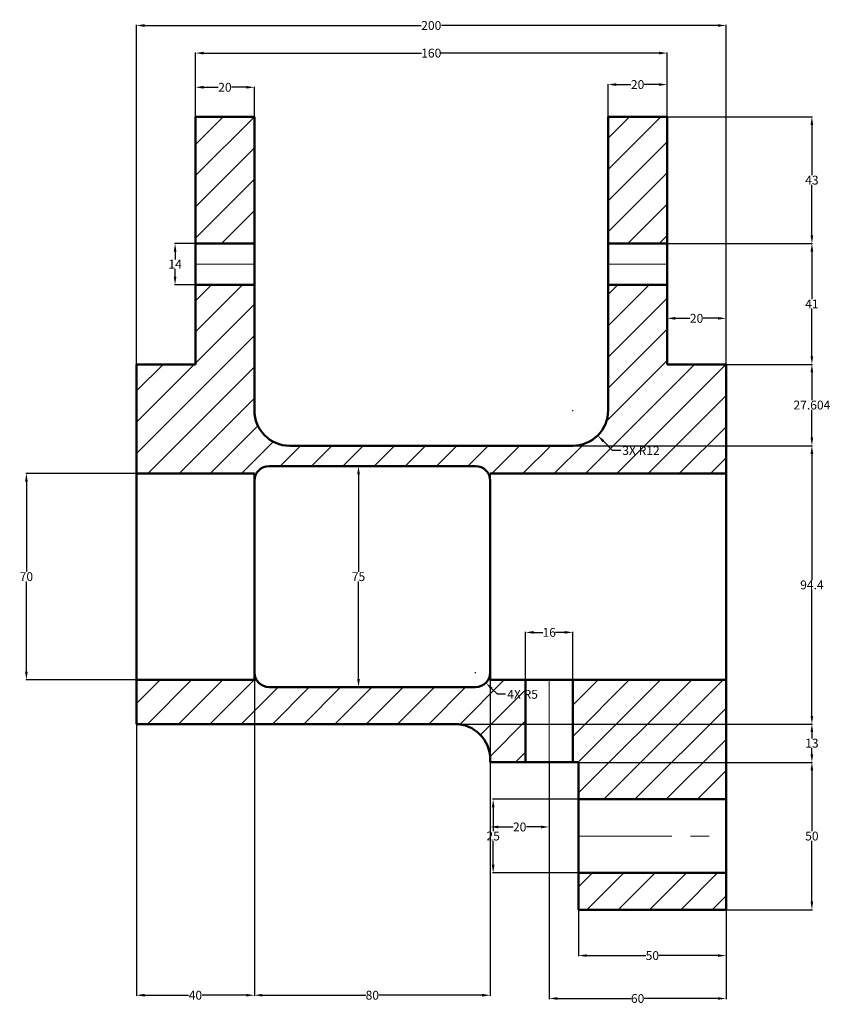
# Model space of a CAD drawing. Units: millimetres. Extents: x 164 to 765, y 152 to 486.
# Tile 2 of 2: x 490 to 765, y 152 to 486. Entities that reach past the tile are written whole.
import ezdxf

# ---------------------------------------------------------------- set-up
doc = ezdxf.new("R2010")
doc.units = ezdxf.units.MM
doc.header["$MEASUREMENT"] = 0
doc.linetypes.add('CENTER', pattern=[50.8, 31.75, -6.35, 6.35, -6.35])
for name, color, linetype, lineweight in [('M-CNTR', 1, 'CENTER', 18), ('M-DIMS', 2, 'Continuous', 25), ('M-HATC', 8, 'Continuous', 18), ('M-OUTL', 7, 'Continuous', 50)]:
    doc.layers.add(name, color=color, linetype=linetype, lineweight=lineweight)
doc.styles.get("Standard").update_dxf_attribs({"font": 'arial.ttf'})
doc.dimstyles.get("Standard").update_dxf_attribs({"dimtxt": 3, "dimasz": 2.75, "dimexe": 0.18, "dimexo": 0.0625, "dimgap": 0.09, "dimtad": 0, "dimtih": 1, "dimtoh": 1, "dimdec": 0, "dimzin": 0, "dimdsep": 46, "dimtxsty": 'Standard', "dimcen": 0.09, "dimadec": 0, "dimazin": 0, "dimtfac": 1, "dimtdec": 0, "dimtofl": 0, "dimtmove": 0, "dimatfit": 3, "dimfxl": 1, "dimtolj": 1, "dimtzin": 0, "dimarcsym": 0})

# ---------------------------------------------------------------- blocks, each defined once
blk = doc.blocks.new('*U11')
at = {"layer": 'M-CNTR', "color": 0, "transparency": 16777216}
blk.add_line((0, 14.12), (0, -14.12), dxfattribs=at)
blk = doc.blocks.new('*U12')
at = {"layer": 'M-CNTR', "color": 0, "transparency": 16777216}
blk.add_line((-25.12, 0), (25.12, 0), dxfattribs=at)
blk = doc.blocks.new('*U13')
at = {"layer": 'M-CNTR', "color": 0, "transparency": 16777216}
blk.add_line((-10.12, 0), (10.12, 0), dxfattribs=at)
blk = doc.blocks.new('*U14')
at = {"layer": 'M-CNTR', "color": 0, "transparency": 16777216}
blk.add_line((-10.12, 0), (10.12, 0), dxfattribs=at)
blk = doc.blocks.new('*D15')
at = {"layer": 'Defpoints', "color": 0, "transparency": 16777216}
for p in [(529.33, 331.64), (491.99, 261.64), (529.33, 261.64)]:
    blk.add_point(p, dxfattribs=at)
at = {"layer": 'M-DIMS', "color": 0, "lineweight": -2, "transparency": 16777216}
for p, q in [((529.27, 331.64), (491.81, 331.64)), ((491.99, 328.89), (491.99, 298.26)), ((491.99, 264.39), (491.99, 295.02)), ((529.27, 261.64), (491.81, 261.64))]:
    blk.add_line(p, q, dxfattribs=at)
at = {"layer": 'M-DIMS', "color": 0, "transparency": 16777216}
for points in [[(491.53, 328.89), (492.45, 328.89), (491.99, 331.64)], [(491.53, 264.39), (492.45, 264.39), (491.99, 261.64)]]:
    blk.add_solid(points, dxfattribs=at)
at = {"layer": 'M-DIMS', "color": 0, "transparency": 16777216, "insert": (491.99, 296.64), "char_height": 3, "attachment_point": 5}
blk.add_mtext('\\A1;70', dxfattribs=at)
blk = doc.blocks.new('*D16')
at = {"layer": 'Defpoints', "color": 0, "transparency": 16777216}
for p in [(604.66, 334.14), (609.33, 334.14), (609.33, 259.14)]:
    blk.add_point(p, dxfattribs=at)
at = {"layer": 'M-DIMS', "color": 0, "lineweight": -2, "transparency": 16777216}
for p, q in [((609.27, 334.14), (604.48, 334.14)), ((604.66, 331.39), (604.66, 298.26)), ((604.66, 261.89), (604.66, 295.03)), ((609.27, 259.14), (604.48, 259.14))]:
    blk.add_line(p, q, dxfattribs=at)
at = {"layer": 'M-DIMS', "color": 0, "transparency": 16777216}
for points in [[(604.2, 331.39), (605.11, 331.39), (604.66, 334.14)], [(604.2, 261.89), (605.11, 261.89), (604.66, 259.14)]]:
    blk.add_solid(points, dxfattribs=at)
at = {"layer": 'M-DIMS', "color": 0, "transparency": 16777216, "insert": (604.66, 296.64), "char_height": 3, "attachment_point": 5}
blk.add_mtext('\\A1;75', dxfattribs=at)
blk = doc.blocks.new('*D17')
at = {"layer": 'Defpoints', "color": 0, "transparency": 16777216}
for p in [(679.33, 183.64), (729.33, 183.64), (729.33, 168.09)]:
    blk.add_point(p, dxfattribs=at)
at = {"layer": 'M-DIMS', "color": 0, "lineweight": -2, "transparency": 16777216}
for p, q in [((679.33, 183.58), (679.33, 167.91)), ((729.33, 183.58), (729.33, 167.91)), ((682.08, 168.09), (702.1, 168.09)), ((726.58, 168.09), (706.56, 168.09))]:
    blk.add_line(p, q, dxfattribs=at)
at = {"layer": 'M-DIMS', "color": 0, "transparency": 16777216}
for points in [[(682.08, 168.55), (682.08, 167.63), (679.33, 168.09)], [(726.58, 168.55), (726.58, 167.63), (729.33, 168.09)]]:
    blk.add_solid(points, dxfattribs=at)
at = {"layer": 'M-DIMS', "color": 0, "transparency": 16777216, "insert": (704.33, 168.09), "char_height": 3, "attachment_point": 5}
blk.add_mtext('\\A1;50', dxfattribs=at)
blk = doc.blocks.new('*D18')
at = {"layer": 'Defpoints', "color": 0, "transparency": 16777216}
for p in [(669.33, 233.52), (729.33, 233.52), (729.33, 153.53)]:
    blk.add_point(p, dxfattribs=at)
at = {"layer": 'M-DIMS', "color": 0, "lineweight": -2, "transparency": 16777216}
for p, q in [((669.33, 233.46), (669.33, 153.35)), ((729.33, 233.46), (729.33, 153.35)), ((672.08, 153.53), (697.09, 153.53)), ((726.58, 153.53), (701.57, 153.53))]:
    blk.add_line(p, q, dxfattribs=at)
at = {"layer": 'M-DIMS', "color": 0, "transparency": 16777216}
for points in [[(672.08, 153.99), (672.08, 153.07), (669.33, 153.53)], [(726.58, 153.99), (726.58, 153.07), (729.33, 153.53)]]:
    blk.add_solid(points, dxfattribs=at)
at = {"layer": 'M-DIMS', "color": 0, "transparency": 16777216, "insert": (699.33, 153.53), "char_height": 3, "attachment_point": 5}
blk.add_mtext('\\A1;60', dxfattribs=at)
blk = doc.blocks.new('*D19')
at = {"layer": 'Defpoints', "color": 0, "transparency": 16777216}
for p in [(649.33, 233.64), (669.33, 233.52), (669.33, 211.71)]:
    blk.add_point(p, dxfattribs=at)
at = {"layer": 'M-DIMS', "color": 0, "lineweight": -2, "transparency": 16777216}
for p, q in [((649.33, 233.58), (649.33, 211.53)), ((669.33, 233.46), (669.33, 211.53)), ((652.08, 211.71), (657.07, 211.71)), ((666.58, 211.71), (661.59, 211.71))]:
    blk.add_line(p, q, dxfattribs=at)
at = {"layer": 'M-DIMS', "color": 0, "transparency": 16777216}
for points in [[(652.08, 212.17), (652.08, 211.25), (649.33, 211.71)], [(666.58, 212.17), (666.58, 211.25), (669.33, 211.71)]]:
    blk.add_solid(points, dxfattribs=at)
at = {"layer": 'M-DIMS', "color": 0, "transparency": 16777216, "insert": (659.33, 211.71), "char_height": 3, "attachment_point": 5}
blk.add_mtext('\\A1;20', dxfattribs=at)
blk = doc.blocks.new('*D20')
at = {"layer": 'Defpoints', "color": 0, "transparency": 16777216}
for p in [(677.33, 277.73), (661.33, 261.64), (677.33, 261.64)]:
    blk.add_point(p, dxfattribs=at)
at = {"layer": 'M-DIMS', "color": 0, "lineweight": -2, "transparency": 16777216}
for p, q in [((661.33, 261.71), (661.33, 277.91)), ((664.08, 277.73), (667.23, 277.73)), ((674.58, 277.73), (671.43, 277.73)), ((677.33, 261.71), (677.33, 277.91))]:
    blk.add_line(p, q, dxfattribs=at)
at = {"layer": 'M-DIMS', "color": 0, "transparency": 16777216}
for points in [[(664.08, 278.19), (664.08, 277.27), (661.33, 277.73)], [(674.58, 278.19), (674.58, 277.27), (677.33, 277.73)]]:
    blk.add_solid(points, dxfattribs=at)
at = {"layer": 'M-DIMS', "color": 0, "transparency": 16777216, "insert": (669.33, 277.73), "char_height": 3, "attachment_point": 5}
blk.add_mtext('\\A1;16', dxfattribs=at)
blk = doc.blocks.new('*D21')
at = {"layer": 'Defpoints', "color": 0, "transparency": 16777216}
for p in [(529.33, 483.59), (529.33, 368.64), (729.33, 368.64)]:
    blk.add_point(p, dxfattribs=at)
at = {"layer": 'M-DIMS', "color": 0, "lineweight": -2, "transparency": 16777216}
for p, q in [((529.33, 368.71), (529.33, 483.77)), ((532.08, 483.59), (625.9, 483.59)), ((726.58, 483.59), (632.75, 483.59)), ((729.33, 368.71), (729.33, 483.77))]:
    blk.add_line(p, q, dxfattribs=at)
at = {"layer": 'M-DIMS', "color": 0, "transparency": 16777216}
for points in [[(532.08, 484.05), (532.08, 483.13), (529.33, 483.59)], [(726.58, 484.05), (726.58, 483.13), (729.33, 483.59)]]:
    blk.add_solid(points, dxfattribs=at)
at = {"layer": 'M-DIMS', "color": 0, "transparency": 16777216, "insert": (629.33, 483.59), "char_height": 3, "attachment_point": 5}
blk.add_mtext('\\A1;200', dxfattribs=at)
blk = doc.blocks.new('*D22')
at = {"layer": 'Defpoints', "color": 0, "transparency": 16777216}
for p in [(569.33, 462.63), (549.33, 452.64), (569.33, 452.64)]:
    blk.add_point(p, dxfattribs=at)
at = {"layer": 'M-DIMS', "color": 0, "lineweight": -2, "transparency": 16777216}
for p, q in [((549.33, 452.71), (549.33, 462.81)), ((552.08, 462.63), (557.07, 462.63)), ((566.58, 462.63), (561.59, 462.63)), ((569.33, 452.71), (569.33, 462.81))]:
    blk.add_line(p, q, dxfattribs=at)
at = {"layer": 'M-DIMS', "color": 0, "transparency": 16777216}
for points in [[(552.08, 463.09), (552.08, 462.17), (549.33, 462.63)], [(566.58, 463.09), (566.58, 462.17), (569.33, 462.63)]]:
    blk.add_solid(points, dxfattribs=at)
at = {"layer": 'M-DIMS', "color": 0, "transparency": 16777216, "insert": (559.33, 462.63), "char_height": 3, "attachment_point": 5}
blk.add_mtext('\\A1;20', dxfattribs=at)
blk = doc.blocks.new('*D23')
at = {"layer": 'Defpoints', "color": 0, "transparency": 16777216}
for p in [(709.33, 474.23), (549.33, 452.64), (709.33, 452.64)]:
    blk.add_point(p, dxfattribs=at)
at = {"layer": 'M-DIMS', "color": 0, "lineweight": -2, "transparency": 16777216}
for p, q in [((549.33, 452.71), (549.33, 474.41)), ((709.33, 452.71), (709.33, 474.41)), ((552.08, 474.23), (626.07, 474.23)), ((706.58, 474.23), (632.59, 474.23))]:
    blk.add_line(p, q, dxfattribs=at)
at = {"layer": 'M-DIMS', "color": 0, "transparency": 16777216}
for points in [[(552.08, 474.69), (552.08, 473.77), (549.33, 474.23)], [(706.58, 474.69), (706.58, 473.77), (709.33, 474.23)]]:
    blk.add_solid(points, dxfattribs=at)
at = {"layer": 'M-DIMS', "color": 0, "transparency": 16777216, "insert": (629.33, 474.23), "char_height": 3, "attachment_point": 5}
blk.add_mtext('\\A1;160', dxfattribs=at)
blk = doc.blocks.new('*D24')
at = {"layer": 'Defpoints', "color": 0, "transparency": 16777216}
for p in [(709.33, 463.56), (689.33, 452.64), (709.33, 452.64)]:
    blk.add_point(p, dxfattribs=at)
at = {"layer": 'M-DIMS', "color": 0, "lineweight": -2, "transparency": 16777216}
for p, q in [((689.33, 452.71), (689.33, 463.74)), ((692.08, 463.56), (697.07, 463.56)), ((706.58, 463.56), (701.59, 463.56)), ((709.33, 452.71), (709.33, 463.74))]:
    blk.add_line(p, q, dxfattribs=at)
at = {"layer": 'M-DIMS', "color": 0, "transparency": 16777216}
for points in [[(692.08, 464.02), (692.08, 463.1), (689.33, 463.56)], [(706.58, 464.02), (706.58, 463.1), (709.33, 463.56)]]:
    blk.add_solid(points, dxfattribs=at)
at = {"layer": 'M-DIMS', "color": 0, "transparency": 16777216, "insert": (699.33, 463.56), "char_height": 3, "attachment_point": 5}
blk.add_mtext('\\A1;20', dxfattribs=at)
blk = doc.blocks.new('*D25')
at = {"layer": 'Defpoints', "color": 0, "transparency": 16777216}
for p in [(729.33, 384.26), (709.33, 368.64), (729.33, 368.64)]:
    blk.add_point(p, dxfattribs=at)
at = {"layer": 'M-DIMS', "color": 0, "lineweight": -2, "transparency": 16777216}
for p, q in [((709.33, 368.71), (709.33, 384.44)), ((712.08, 384.26), (717.07, 384.26)), ((726.58, 384.26), (721.59, 384.26)), ((729.33, 368.71), (729.33, 384.44))]:
    blk.add_line(p, q, dxfattribs=at)
at = {"layer": 'M-DIMS', "color": 0, "transparency": 16777216}
for points in [[(712.08, 384.72), (712.08, 383.8), (709.33, 384.26)], [(726.58, 384.72), (726.58, 383.8), (729.33, 384.26)]]:
    blk.add_solid(points, dxfattribs=at)
at = {"layer": 'M-DIMS', "color": 0, "transparency": 16777216, "insert": (719.33, 384.26), "char_height": 3, "attachment_point": 5}
blk.add_mtext('\\A1;20', dxfattribs=at)
blk = doc.blocks.new('*D26')
at = {"layer": 'Defpoints', "color": 0, "transparency": 16777216}
for p in [(569.33, 409.64), (542.43, 395.64), (569.33, 395.64)]:
    blk.add_point(p, dxfattribs=at)
at = {"layer": 'M-DIMS', "color": 0, "lineweight": -2, "transparency": 16777216}
for p, q in [((569.27, 409.64), (542.25, 409.64)), ((542.43, 406.89), (542.43, 404.24)), ((542.43, 398.39), (542.43, 401.05)), ((569.27, 395.64), (542.25, 395.64))]:
    blk.add_line(p, q, dxfattribs=at)
at = {"layer": 'M-DIMS', "color": 0, "transparency": 16777216}
for points in [[(541.97, 406.89), (542.88, 406.89), (542.43, 409.64)], [(541.97, 398.39), (542.88, 398.39), (542.43, 395.64)]]:
    blk.add_solid(points, dxfattribs=at)
at = {"layer": 'M-DIMS', "color": 0, "transparency": 16777216, "insert": (542.43, 402.64), "char_height": 3, "attachment_point": 5}
blk.add_mtext('\\A1;14', dxfattribs=at)
blk = doc.blocks.new('*D28')
at = {"layer": 'Defpoints', "color": 0, "transparency": 16777216}
for p in [(649.33, 233.64), (758.45, 233.64), (729.33, 183.64)]:
    blk.add_point(p, dxfattribs=at)
at = {"layer": 'M-DIMS', "color": 0, "lineweight": -2, "transparency": 16777216}
for p, q in [((649.39, 233.64), (758.63, 233.64)), ((758.45, 230.89), (758.45, 210.26)), ((758.45, 186.39), (758.45, 207.02)), ((729.39, 183.64), (758.63, 183.64))]:
    blk.add_line(p, q, dxfattribs=at)
at = {"layer": 'M-DIMS', "color": 0, "transparency": 16777216}
for points in [[(757.99, 230.89), (758.91, 230.89), (758.45, 233.64)], [(757.99, 186.39), (758.91, 186.39), (758.45, 183.64)]]:
    blk.add_solid(points, dxfattribs=at)
at = {"layer": 'M-DIMS', "color": 0, "transparency": 16777216, "insert": (758.45, 208.64), "char_height": 3, "attachment_point": 5}
blk.add_mtext('\\A1;50', dxfattribs=at)
blk = doc.blocks.new('*D29')
at = {"layer": 'Defpoints', "color": 0, "transparency": 16777216}
for p in [(529.33, 246.64), (758.45, 246.64), (649.33, 233.64)]:
    blk.add_point(p, dxfattribs=at)
at = {"layer": 'M-DIMS', "color": 0, "lineweight": -2, "transparency": 16777216}
for p, q in [((529.39, 246.64), (758.63, 246.64)), ((758.45, 243.89), (758.45, 241.77)), ((758.45, 236.39), (758.45, 238.52)), ((649.39, 233.64), (758.63, 233.64))]:
    blk.add_line(p, q, dxfattribs=at)
at = {"layer": 'M-DIMS', "color": 0, "transparency": 16777216}
for points in [[(757.99, 243.89), (758.91, 243.89), (758.45, 246.64)], [(757.99, 236.39), (758.91, 236.39), (758.45, 233.64)]]:
    blk.add_solid(points, dxfattribs=at)
at = {"layer": 'M-DIMS', "color": 0, "transparency": 16777216, "insert": (758.45, 240.14), "char_height": 3, "attachment_point": 5}
blk.add_mtext('\\A1;13', dxfattribs=at)
blk = doc.blocks.new('*D30')
at = {"layer": 'Defpoints', "color": 0, "transparency": 16777216}
for p in [(677.33, 341.04), (758.45, 341.04), (529.33, 246.64)]:
    blk.add_point(p, dxfattribs=at)
at = {"layer": 'M-DIMS', "color": 0, "lineweight": -2, "transparency": 16777216}
for p, q in [((677.39, 341.04), (758.63, 341.04)), ((758.45, 338.29), (758.45, 295.46)), ((758.45, 249.39), (758.45, 292.22)), ((529.39, 246.64), (758.63, 246.64))]:
    blk.add_line(p, q, dxfattribs=at)
at = {"layer": 'M-DIMS', "color": 0, "transparency": 16777216}
for points in [[(757.99, 338.29), (758.91, 338.29), (758.45, 341.04)], [(757.99, 249.39), (758.91, 249.39), (758.45, 246.64)]]:
    blk.add_solid(points, dxfattribs=at)
at = {"layer": 'M-DIMS', "color": 0, "transparency": 16777216, "insert": (758.45, 293.84), "char_height": 3, "attachment_point": 5}
blk.add_mtext('\\A1;94.4', dxfattribs=at)
blk = doc.blocks.new('*D31')
at = {"layer": 'Defpoints', "color": 0, "transparency": 16777216}
for p in [(729.33, 368.64), (758.45, 368.64), (677.33, 341.04)]:
    blk.add_point(p, dxfattribs=at)
at = {"layer": 'M-DIMS', "color": 0, "lineweight": -2, "transparency": 16777216}
for p, q in [((729.39, 368.64), (758.63, 368.64)), ((758.45, 365.89), (758.45, 356.46)), ((758.45, 343.79), (758.45, 353.22)), ((677.39, 341.04), (758.63, 341.04))]:
    blk.add_line(p, q, dxfattribs=at)
at = {"layer": 'M-DIMS', "color": 0, "transparency": 16777216}
for points in [[(757.99, 365.89), (758.91, 365.89), (758.45, 368.64)], [(757.99, 343.79), (758.91, 343.79), (758.45, 341.04)]]:
    blk.add_solid(points, dxfattribs=at)
at = {"layer": 'M-DIMS', "color": 0, "transparency": 16777216, "insert": (758.45, 354.84), "char_height": 3, "attachment_point": 5}
blk.add_mtext('\\A1;27.604', dxfattribs=at)
blk = doc.blocks.new('*D32')
at = {"layer": 'Defpoints', "color": 0, "transparency": 16777216}
for p in [(709.33, 409.64), (758.45, 409.64), (729.33, 368.64)]:
    blk.add_point(p, dxfattribs=at)
at = {"layer": 'M-DIMS', "color": 0, "lineweight": -2, "transparency": 16777216}
for p, q in [((709.39, 409.64), (758.63, 409.64)), ((758.45, 406.89), (758.45, 390.74)), ((758.45, 371.39), (758.45, 387.55)), ((729.39, 368.64), (758.63, 368.64))]:
    blk.add_line(p, q, dxfattribs=at)
at = {"layer": 'M-DIMS', "color": 0, "transparency": 16777216}
for points in [[(757.99, 406.89), (758.91, 406.89), (758.45, 409.64)], [(757.99, 371.39), (758.91, 371.39), (758.45, 368.64)]]:
    blk.add_solid(points, dxfattribs=at)
at = {"layer": 'M-DIMS', "color": 0, "transparency": 16777216, "insert": (758.45, 389.14), "char_height": 3, "attachment_point": 5}
blk.add_mtext('\\A1;41', dxfattribs=at)
blk = doc.blocks.new('*D33')
at = {"layer": 'Defpoints', "color": 0, "transparency": 16777216}
for p in [(709.33, 452.64), (758.45, 452.64), (709.33, 409.64)]:
    blk.add_point(p, dxfattribs=at)
at = {"layer": 'M-DIMS', "color": 0, "lineweight": -2, "transparency": 16777216}
for p, q in [((709.39, 452.64), (758.63, 452.64)), ((758.45, 449.89), (758.45, 432.77)), ((758.45, 412.39), (758.45, 429.52)), ((709.39, 409.64), (758.63, 409.64))]:
    blk.add_line(p, q, dxfattribs=at)
at = {"layer": 'M-DIMS', "color": 0, "transparency": 16777216}
for points in [[(757.99, 449.89), (758.91, 449.89), (758.45, 452.64)], [(757.99, 412.39), (758.91, 412.39), (758.45, 409.64)]]:
    blk.add_solid(points, dxfattribs=at)
at = {"layer": 'M-DIMS', "color": 0, "transparency": 16777216, "insert": (758.45, 431.14), "char_height": 3, "attachment_point": 5}
blk.add_mtext('\\A1;43', dxfattribs=at)
blk = doc.blocks.new('*D34')
at = {"layer": 'Defpoints', "color": 0, "transparency": 16777216}
for p in [(650.33, 221.14), (679.33, 221.14), (679.33, 196.14)]:
    blk.add_point(p, dxfattribs=at)
at = {"layer": 'M-DIMS', "color": 0, "lineweight": -2, "transparency": 16777216}
for p, q in [((679.27, 221.14), (650.15, 221.14)), ((650.33, 218.39), (650.33, 210.26)), ((650.33, 198.89), (650.33, 207.02)), ((679.27, 196.14), (650.15, 196.14))]:
    blk.add_line(p, q, dxfattribs=at)
at = {"layer": 'M-DIMS', "color": 0, "transparency": 16777216}
for points in [[(649.87, 218.39), (650.79, 218.39), (650.33, 221.14)], [(649.87, 198.89), (650.79, 198.89), (650.33, 196.14)]]:
    blk.add_solid(points, dxfattribs=at)
at = {"layer": 'M-DIMS', "color": 0, "transparency": 16777216, "insert": (650.33, 208.64), "char_height": 3, "attachment_point": 5}
blk.add_mtext('\\A1;25', dxfattribs=at)
blk = doc.blocks.new('*D35')
at = {"layer": 'Defpoints', "color": 0, "transparency": 16777216}
for p in [(529.33, 331.64), (569.33, 331.64), (569.33, 154.64)]:
    blk.add_point(p, dxfattribs=at)
at = {"layer": 'M-DIMS', "color": 0, "lineweight": -2, "transparency": 16777216}
for p, q in [((529.33, 331.58), (529.33, 154.46)), ((569.33, 331.58), (569.33, 154.46)), ((532.08, 154.64), (547.03, 154.64)), ((566.58, 154.64), (551.62, 154.64))]:
    blk.add_line(p, q, dxfattribs=at)
at = {"layer": 'M-DIMS', "color": 0, "transparency": 16777216}
for points in [[(532.08, 155.1), (532.08, 154.18), (529.33, 154.64)], [(566.58, 155.1), (566.58, 154.18), (569.33, 154.64)]]:
    blk.add_solid(points, dxfattribs=at)
at = {"layer": 'M-DIMS', "color": 0, "transparency": 16777216, "insert": (549.33, 154.64), "char_height": 3, "attachment_point": 5}
blk.add_mtext('\\A1;40', dxfattribs=at)
blk = doc.blocks.new('*D36')
at = {"layer": 'Defpoints', "color": 0, "transparency": 16777216}
for p in [(569.33, 331.64), (649.33, 331.64), (649.33, 154.64)]:
    blk.add_point(p, dxfattribs=at)
at = {"layer": 'M-DIMS', "color": 0, "lineweight": -2, "transparency": 16777216}
for p, q in [((569.33, 331.58), (569.33, 154.46)), ((649.33, 331.58), (649.33, 154.46)), ((572.08, 154.64), (607.09, 154.64)), ((646.58, 154.64), (611.56, 154.64))]:
    blk.add_line(p, q, dxfattribs=at)
at = {"layer": 'M-DIMS', "color": 0, "transparency": 16777216}
for points in [[(572.08, 155.1), (572.08, 154.18), (569.33, 154.64)], [(646.58, 155.1), (646.58, 154.18), (649.33, 154.64)]]:
    blk.add_solid(points, dxfattribs=at)
at = {"layer": 'M-DIMS', "color": 0, "transparency": 16777216, "insert": (609.33, 154.64), "char_height": 3, "attachment_point": 5}
blk.add_mtext('\\A1;80', dxfattribs=at)
blk = doc.blocks.new('*D41')
at = {"layer": 'Defpoints', "color": 0, "transparency": 16777216}
for p in [(677.33, 353.04), (685.78, 344.52)]:
    blk.add_point(p, dxfattribs=at)
at = {"layer": 'M-DIMS', "color": 0, "lineweight": -2, "transparency": 16777216}
for p, q in [((677.24, 353.04), (677.42, 353.04)), ((677.33, 352.95), (677.33, 353.13)), ((690.85, 339.41), (687.72, 342.57)), ((693.6, 339.41), (690.85, 339.41))]:
    blk.add_line(p, q, dxfattribs=at)
at = {"layer": 'M-DIMS', "color": 0, "transparency": 16777216}
blk.add_solid([(688.04, 342.89), (687.39, 342.24), (685.78, 344.52)], dxfattribs=at)
at = {"layer": 'M-DIMS', "color": 0, "transparency": 16777216, "insert": (700.48, 339.41), "char_height": 3, "attachment_point": 5}
blk.add_mtext('\\A1;3X R12', dxfattribs=at)
blk = doc.blocks.new('*D42')
at = {"layer": 'Defpoints', "color": 0, "transparency": 16777216}
for p in [(644.33, 264.14), (647.86, 260.61)]:
    blk.add_point(p, dxfattribs=at)
at = {"layer": 'M-DIMS', "color": 0, "lineweight": -2, "transparency": 16777216}
for p, q in [((644.24, 264.14), (644.42, 264.14)), ((644.33, 264.05), (644.33, 264.23)), ((651.75, 256.72), (649.81, 258.66)), ((654.5, 256.72), (651.75, 256.72))]:
    blk.add_line(p, q, dxfattribs=at)
at = {"layer": 'M-DIMS', "color": 0, "transparency": 16777216}
blk.add_solid([(650.13, 258.99), (649.48, 258.34), (647.86, 260.61)], dxfattribs=at)
at = {"layer": 'M-DIMS', "color": 0, "transparency": 16777216, "insert": (660.31, 256.72), "char_height": 3, "attachment_point": 5}
blk.add_mtext('\\A1;4X R5', dxfattribs=at)

msp = doc.modelspace()

# ---------------------------------------------------------------- hatches: boundary and pattern name
at = {"layer": 'M-HATC'}
h = msp.add_hatch(dxfattribs=at)
h.set_pattern_fill('ANSI31', color=256, scale=60)
h.paths.add_polyline_path([(569.329, 452.6431), (549.329, 452.6431), (549.329, 409.6431), (569.329, 409.6431)])
h.paths.add_polyline_path([(709.329, 452.6431), (689.329, 452.6431), (689.329, 409.6431), (709.329, 409.6431)])
h.paths.add_polyline_path([(729.329, 196.1431), (679.329, 196.1431), (679.329, 183.6431), (729.329, 183.6431)])
h.paths.add_polyline_path([(729.329, 261.6431), (677.329, 261.6431), (677.329, 233.6431), (679.329, 233.6431), (679.329, 221.1431), (729.329, 221.1431)])
h = msp.add_hatch(dxfattribs=at)
h.set_pattern_fill('ANSI31', color=256, scale=60)
h.paths.add_polyline_path([(661.329, 261.6431), (649.329, 261.6431), (649.329, 259.1431), (569.329, 259.1431), (569.329, 261.6431), (529.329, 261.6431), (529.329, 246.6431), (637.329, 246.6431, -0.41421356), (649.329, 234.6431), (649.329, 233.6431), (661.329, 233.6431)])
h.paths.add_polyline_path([(569.329, 353.039), (569.329, 395.6431), (549.329, 395.6431), (549.329, 368.6431), (529.329, 368.6431), (529.329, 331.6431), (569.329, 331.6431), (569.329, 334.1431), (649.329, 334.1431), (649.329, 331.6431), (729.329, 331.6431), (729.329, 368.6431), (709.329, 368.6431), (709.329, 395.6431), (689.329, 395.6431), (689.329, 353.039, -0.41421356), (677.329, 341.039), (581.329, 341.039, -0.41421356)])

# ---------------------------------------------------------------- linework, layer by layer
at = {"layer": 'M-OUTL'}
for p, q in [((549.329, 452.6431), (549.329, 368.6431)), ((569.329, 452.6431), (549.329, 452.6431)), ((569.329, 452.6431), (569.329, 352.6431)), ((689.329, 452.6431), (689.329, 352.6431)), ((689.329, 452.6431), (709.329, 452.6431)), ((709.329, 452.6431), (709.329, 368.6431)), ((549.329, 409.6431), (569.329, 409.6431)), ((689.329, 409.6431), (709.329, 409.6431)), ((549.329, 395.6431), (569.329, 395.6431)), ((689.329, 395.6431), (709.329, 395.6431)), ((529.329, 368.6431), (529.329, 246.6431)), ((529.329, 368.6431), (549.329, 368.6431)), ((709.329, 368.6431), (729.329, 368.6431)), ((709.329, 368.6431), (729.329, 368.6431)), ((729.329, 368.6431), (729.329, 183.6431)), ((581.329, 341.039), (677.329, 341.039)), ((574.329, 334.1431), (644.329, 334.1431)), ((529.329, 331.6431), (569.329, 331.6431)), ((569.329, 331.6431), (569.329, 261.6431)), ((649.329, 331.6431), (729.329, 331.6431)), ((649.329, 329.1431), (649.329, 261.6431)), ((649.329, 261.6431), (649.329, 329.1431)), ((529.329, 261.6431), (569.329, 261.6431)), ((649.329, 261.6431), (729.329, 261.6431)), ((661.329, 261.6431), (661.329, 233.6431)), ((677.329, 261.6431), (677.329, 233.6431)), ((574.329, 259.1431), (644.329, 259.1431)), ((529.329, 246.6431), (637.329, 246.6431)), ((649.329, 233.6431), (649.329, 234.6431)), ((669.329, 233.6431), (649.329, 233.6431)), ((679.329, 233.6431), (659.329, 233.6431)), ((679.329, 233.6431), (679.329, 183.6431)), ((679.329, 221.1431), (729.329, 221.1431)), ((679.329, 196.1431), (729.329, 196.1431)), ((679.329, 183.6431), (729.329, 183.6431))]:
    msp.add_line(p, q, dxfattribs=at)
for centre, radius, start, end in [((581.329, 353.039), 12, 180, 270), ((677.329, 353.039), 12, 270, 360), ((574.329, 329.1431), 5, 90, 180), ((644.329, 329.1431), 5, 0, 90), ((574.329, 264.1431), 5, 180, 270), ((644.329, 264.1431), 5, 270, 0), ((637.329, 234.6431), 12, 0, 90)]:
    msp.add_arc(centre, radius, start, end, dxfattribs=at)

# ---------------------------------------------------------------- block references
at = {"layer": 'M-CNTR'}
for name, p in [('*U14', (559.329, 402.6431)), ('*U13', (699.329, 402.6431)), ('*U11', (669.329, 247.6431)), ('*U12', (704.329, 208.6431))]:
    msp.add_blockref(name, p, dxfattribs=at)

# ---------------------------------------------------------------- dimensions: what is measured, and where the dimension line sits
at = {"layer": 'M-DIMS'}
for base, p1, p2, override, picture, middle in [((529.329, 483.592), (729.329, 368.6431), (529.329, 368.6431), {"dimclrd": 0, "dimclre": 0, "dimclrt": 0}, '*D21', (629.329, 483.592)), ((709.329, 474.2333), (549.329, 452.6431), (709.329, 452.6431), {"dimclrd": 0, "dimclre": 0, "dimclrt": 0}, '*D23', (629.329, 474.2333)), ((569.329, 462.6319), (549.329, 452.6431), (569.329, 452.6431), {"dimclrd": 0, "dimclre": 0, "dimclrt": 0}, '*D22', (559.329, 462.6319)), ((709.329, 463.5594), (689.329, 452.6431), (709.329, 452.6431), {"dimclrd": 0, "dimclre": 0, "dimclrt": 0}, '*D24', (699.329, 463.5594)), ((729.329, 384.2574), (709.329, 368.6431), (729.329, 368.6431), {"dimclrd": 0, "dimclre": 0, "dimclrt": 0}, '*D25', (719.329, 384.2574)), ((569.329, 154.6431), (529.329, 331.6431), (569.329, 331.6431), {"dimdec": 0, "dimlfac": 1, "dimrnd": 0, "dimzin": 0, "dimdsep": 46, "dimlunit": 2}, '*D35', (549.329, 154.6431)), ((649.329, 154.6431), (569.329, 331.6431), (649.329, 331.6431), {"dimdec": 0, "dimlfac": 1, "dimrnd": 0, "dimzin": 0, "dimdsep": 46, "dimlunit": 2}, '*D36', (609.329, 154.6431)), ((677.329, 277.7281), (661.329, 261.6431), (677.329, 261.6431), {"dimclrd": 0, "dimclre": 0, "dimclrt": 0}, '*D20', (669.329, 277.7281)), ((669.329, 211.7079), (649.329, 233.6431), (669.329, 233.5231), {"dimclrd": 0, "dimclre": 0, "dimclrt": 0}, '*D19', (659.329, 211.7079)), ((729.329, 153.5276), (669.329, 233.5231), (729.329, 233.5231), {"dimclrd": 0, "dimclre": 0, "dimclrt": 0}, '*D18', (699.329, 153.5276)), ((729.329, 168.0899), (679.329, 183.6431), (729.329, 183.6431), {"dimclrd": 0, "dimclre": 0, "dimclrt": 0}, '*D17', (704.329, 168.0899))]:
    dim = msp.add_linear_dim(base=base, p1=p1, p2=p2, dimstyle='Standard', override=override, dxfattribs=at)
    dim.commit()
    dim.dimension.update_dxf_attribs({"geometry": picture, "text_midpoint": middle})
for base, p1, p2, override, picture, middle in [((758.449, 452.6431), (709.329, 409.6431), (709.329, 452.6431), {"dimdec": 0, "dimlfac": 1, "dimrnd": 0, "dimzin": 0, "dimdsep": 46, "dimlunit": 2}, '*D33', (758.449, 431.1431)), ((542.4257, 395.6431), (569.329, 409.6431), (569.329, 395.6431), {"dimclrd": 0, "dimclre": 0, "dimclrt": 0}, '*D26', (542.4257, 402.6431)), ((758.449, 409.6431), (729.329, 368.6431), (709.329, 409.6431), {"dimdec": 0, "dimlfac": 1, "dimrnd": 0, "dimzin": 0, "dimdsep": 46, "dimlunit": 2}, '*D32', (758.449, 389.1431)), ((758.449, 368.6431), (677.329, 341.039), (729.329, 368.6431), {"dimdec": 3, "dimlfac": 1, "dimrnd": 0, "dimzin": 0, "dimdsep": 46, "dimlunit": 2}, '*D31', (758.449, 354.841)), ((758.449, 341.039), (529.329, 246.6431), (677.329, 341.039), {"dimdec": 1, "dimlfac": 1, "dimrnd": 0, "dimzin": 0, "dimdsep": 46, "dimlunit": 2}, '*D30', (758.449, 293.841)), ((604.6554, 334.1431), (609.329, 259.1431), (609.329, 334.1431), {"dimclrd": 0, "dimclre": 0, "dimclrt": 0}, '*D16', (604.6554, 296.6431)), ((491.9873, 261.6431), (529.329, 331.6431), (529.329, 261.6431), {"dimclrd": 0, "dimclre": 0, "dimclrt": 0}, '*D15', (491.9873, 296.6431)), ((758.449, 246.6431), (649.329, 233.6431), (529.329, 246.6431), {"dimdec": 0, "dimlfac": 1, "dimrnd": 0, "dimzin": 0, "dimdsep": 46, "dimlunit": 2}, '*D29', (758.449, 240.1431)), ((758.449, 233.6431), (729.329, 183.6431), (649.329, 233.6431), {"dimdec": 0, "dimlfac": 1, "dimrnd": 0, "dimzin": 0, "dimdsep": 46, "dimlunit": 2}, '*D28', (758.449, 208.6431)), ((650.329, 221.1431), (679.329, 196.1431), (679.329, 221.1431), {"dimdec": 0, "dimlfac": 1, "dimrnd": 0, "dimzin": 0, "dimdsep": 46, "dimlunit": 2}, '*D34', (650.329, 208.6431))]:
    dim = msp.add_linear_dim(base=base, p1=p1, p2=p2, angle=90, dimstyle='Standard', override=override, dxfattribs=at)
    dim.commit()
    dim.dimension.update_dxf_attribs({"geometry": picture, "text_midpoint": middle})
dim = msp.add_radius_dim(center=(677.329, 353.039), mpoint=(685.7803, 344.5199), text='3X <>', dimstyle='Standard', override={"dimdec": 0, "dimlfac": 1, "dimrnd": 0, "dimzin": 0, "dimdsep": 46, "dimlunit": 2}, dxfattribs=at)
dim.commit()
dim.dimension.update_dxf_attribs({"geometry": '*D41', "text_midpoint": (700.482, 339.4084), "dimtype": 164})
dim = msp.add_radius_dim(center=(644.329, 264.1431), mpoint=(647.8645, 260.6075), text='4X <>', dimstyle='Standard', override={"dimdec": 0, "dimlfac": 1, "dimrnd": 0, "dimzin": 0, "dimdsep": 46, "dimlunit": 2}, dxfattribs=at)
dim.commit()
dim.dimension.update_dxf_attribs({"geometry": '*D42', "text_midpoint": (660.3071, 256.7184)})

doc.saveas('drawing.dxf')
